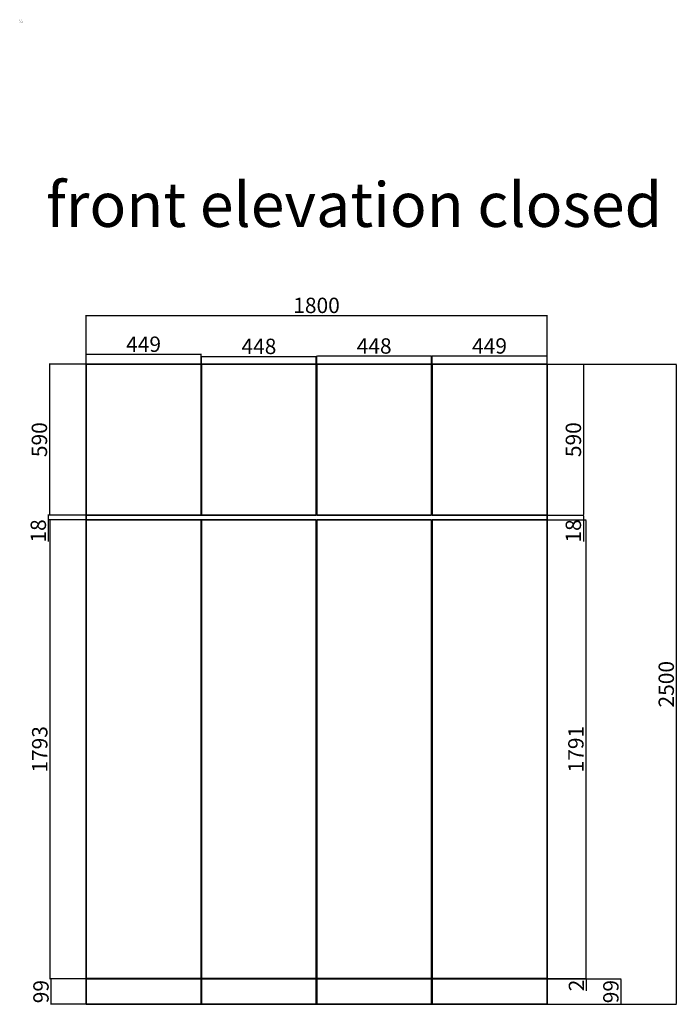
# Model space of a CAD drawing. Units: millimetres. Extents: x 222 to 5960, y 495 to 4622.
# Tile 3 of 3: x 3388 to 5960, y 776 to 4622. Entities that reach past the tile are written whole.
import ezdxf

# ---------------------------------------------------------------- set-up
doc = ezdxf.new("R2010")
doc.units = ezdxf.units.MM
for name, color, linetype, lineweight in [('A-ANNO-DIMS', 2, 'Continuous', 18), ('A-ANNO-TEXT', 3, 'Continuous', 25), ('A-FURN', 7, 'Continuous', 35)]:
    doc.layers.add(name, color=color, linetype=linetype, lineweight=lineweight)
doc.styles.get("Standard").update_dxf_attribs({"font": 'arial.ttf'})
doc.dimstyles.new('ISO-25', dxfattribs={"dimtxt": 60, "dimasz": 2.5, "dimexe": 1.25, "dimexo": 0.625, "dimtad": 1, "dimtxsty": 'Standard', "dimcen": 2.5, "dimadec": 0, "dimazin": 0, "dimtfac": 1, "dimtmove": 0, "dimatfit": 3, "dimfxl": 1, "dimarcsym": 0})

# ---------------------------------------------------------------- blocks, each defined once
blk = doc.blocks.new('*D38')
at = {"layer": 'A-ANNO-DIMS', "color": 0, "lineweight": -2, "transparency": 16777216}
for p, q in [((3647.7, 3277), (3647.7, 3316.4)), ((3650.2, 3315.2), (4094.2, 3315.2)), ((4096.7, 3277), (4096.7, 3316.4))]:
    blk.add_line(p, q, dxfattribs=at)
at = {"layer": 'A-ANNO-DIMS', "color": 0, "transparency": 16777216}
for points in [[(3650.2, 3315.6), (3650.2, 3314.8), (3647.7, 3315.2)], [(4094.2, 3315.6), (4094.2, 3314.8), (4096.7, 3315.2)]]:
    blk.add_solid(points, dxfattribs=at)
at = {"layer": 'Defpoints', "color": 0, "transparency": 16777216}
for p in [(4096.7, 3315.2), (3647.7, 3276.4), (4096.7, 3276.4)]:
    blk.add_point(p, dxfattribs=at)
at = {"layer": 'A-ANNO-DIMS', "color": 0, "transparency": 16777216, "insert": (3872.2, 3346.4), "char_height": 60, "attachment_point": 5}
blk.add_mtext('449', dxfattribs=at)
blk = doc.blocks.new('*D39')
at = {"layer": 'A-ANNO-DIMS', "color": 0, "lineweight": -2, "transparency": 16777216}
for p, q in [((4098.7, 3277), (4098.7, 3308)), ((4546.7, 3277), (4546.7, 3308)), ((4101.2, 3306.7), (4544.2, 3306.7))]:
    blk.add_line(p, q, dxfattribs=at)
at = {"layer": 'A-ANNO-DIMS', "color": 0, "transparency": 16777216}
for points in [[(4101.2, 3307.1), (4101.2, 3306.3), (4098.7, 3306.7)], [(4544.2, 3307.1), (4544.2, 3306.3), (4546.7, 3306.7)]]:
    blk.add_solid(points, dxfattribs=at)
at = {"layer": 'Defpoints', "color": 0, "transparency": 16777216}
for p in [(4098.7, 3276.4), (4546.7, 3306.7), (4546.7, 3276.4)]:
    blk.add_point(p, dxfattribs=at)
at = {"layer": 'A-ANNO-DIMS', "color": 0, "transparency": 16777216, "insert": (4322.7, 3338), "char_height": 60, "attachment_point": 5}
blk.add_mtext('448', dxfattribs=at)
blk = doc.blocks.new('*D40')
at = {"layer": 'A-ANNO-DIMS', "color": 0, "lineweight": -2, "transparency": 16777216}
for p, q in [((4548.7, 3277), (4548.7, 3309.4)), ((4551.2, 3308.2), (4994.2, 3308.2)), ((4996.7, 3277), (4996.7, 3309.4))]:
    blk.add_line(p, q, dxfattribs=at)
at = {"layer": 'A-ANNO-DIMS', "color": 0, "transparency": 16777216}
for points in [[(4551.2, 3308.6), (4551.2, 3307.8), (4548.7, 3308.2)], [(4994.2, 3308.6), (4994.2, 3307.8), (4996.7, 3308.2)]]:
    blk.add_solid(points, dxfattribs=at)
at = {"layer": 'Defpoints', "color": 0, "transparency": 16777216}
for p in [(4996.7, 3308.2), (4548.7, 3276.4), (4996.7, 3276.4)]:
    blk.add_point(p, dxfattribs=at)
at = {"layer": 'A-ANNO-DIMS', "color": 0, "transparency": 16777216, "insert": (4772.7, 3339.5), "char_height": 60, "attachment_point": 5}
blk.add_mtext('448', dxfattribs=at)
blk = doc.blocks.new('*D41')
at = {"layer": 'A-ANNO-DIMS', "color": 0, "lineweight": -2, "transparency": 16777216}
for p, q in [((4998.7, 3277), (4998.7, 3309.7)), ((5001.2, 3308.5), (5445.2, 3308.5)), ((5447.7, 3277), (5447.7, 3309.7))]:
    blk.add_line(p, q, dxfattribs=at)
at = {"layer": 'A-ANNO-DIMS', "color": 0, "transparency": 16777216}
for points in [[(5001.2, 3308.9), (5001.2, 3308.1), (4998.7, 3308.5)], [(5445.2, 3308.9), (5445.2, 3308.1), (5447.7, 3308.5)]]:
    blk.add_solid(points, dxfattribs=at)
at = {"layer": 'Defpoints', "color": 0, "transparency": 16777216}
for p in [(5447.7, 3308.5), (4998.7, 3276.4), (5447.7, 3276.4)]:
    blk.add_point(p, dxfattribs=at)
at = {"layer": 'A-ANNO-DIMS', "color": 0, "transparency": 16777216, "insert": (5223.2, 3339.7), "char_height": 60, "attachment_point": 5}
blk.add_mtext('449', dxfattribs=at)
blk = doc.blocks.new('*D42')
at = {"layer": 'A-ANNO-DIMS', "color": 0, "lineweight": -2, "transparency": 16777216}
for p, q in [((3647.7, 3277), (3647.7, 3468)), ((3650.2, 3466.7), (5445.2, 3466.7)), ((5447.7, 3277), (5447.7, 3468))]:
    blk.add_line(p, q, dxfattribs=at)
at = {"layer": 'A-ANNO-DIMS', "color": 0, "transparency": 16777216}
for points in [[(3650.2, 3467.1), (3650.2, 3466.3), (3647.7, 3466.7)], [(5445.2, 3467.1), (5445.2, 3466.3), (5447.7, 3466.7)]]:
    blk.add_solid(points, dxfattribs=at)
at = {"layer": 'Defpoints', "color": 0, "transparency": 16777216}
for p in [(5447.7, 3466.7), (3647.7, 3276.4), (5447.7, 3276.4)]:
    blk.add_point(p, dxfattribs=at)
at = {"layer": 'A-ANNO-DIMS', "color": 0, "transparency": 16777216, "insert": (4547.7, 3498), "char_height": 60, "attachment_point": 5}
blk.add_mtext('1800', dxfattribs=at)
blk = doc.blocks.new('*D43')
at = {"layer": 'A-ANNO-DIMS', "color": 0, "lineweight": -2, "transparency": 16777216}
for p, q in [((5448.4, 3276.4), (5591, 3276.4)), ((5589.7, 3273.9), (5589.7, 2688.9)), ((5448.4, 2686.4), (5591, 2686.4))]:
    blk.add_line(p, q, dxfattribs=at)
at = {"layer": 'A-ANNO-DIMS', "color": 0, "transparency": 16777216}
for points in [[(5589.3, 3273.9), (5590.2, 3273.9), (5589.7, 3276.4)], [(5589.3, 2688.9), (5590.2, 2688.9), (5589.7, 2686.4)]]:
    blk.add_solid(points, dxfattribs=at)
at = {"layer": 'Defpoints', "color": 0, "transparency": 16777216}
for p in [(5447.7, 3276.4), (5447.7, 2686.4), (5589.7, 2686.4)]:
    blk.add_point(p, dxfattribs=at)
at = {"layer": 'A-ANNO-DIMS', "color": 0, "transparency": 16777216, "insert": (5558.5, 2981.4), "char_height": 60, "attachment_point": 5, "rotation": 90}
blk.add_mtext('590', dxfattribs=at)
blk = doc.blocks.new('*D44')
at = {"layer": 'A-ANNO-DIMS', "color": 0, "lineweight": -2, "transparency": 16777216}
for p, q in [((5448.4, 2686.4), (5590.8, 2686.4)), ((5448.4, 2668.4), (5590.8, 2668.4)), ((5589.6, 2683.9), (5589.6, 2670.9)), ((5589.6, 2668.4), (5589.6, 2584.2))]:
    blk.add_line(p, q, dxfattribs=at)
at = {"layer": 'A-ANNO-DIMS', "color": 0, "transparency": 16777216}
for points in [[(5589.1, 2683.9), (5590, 2683.9), (5589.6, 2686.4)], [(5589.1, 2670.9), (5590, 2670.9), (5589.6, 2668.4)]]:
    blk.add_solid(points, dxfattribs=at)
at = {"layer": 'Defpoints', "color": 0, "transparency": 16777216}
for p in [(5447.7, 2686.4), (5447.7, 2668.4), (5589.6, 2668.4)]:
    blk.add_point(p, dxfattribs=at)
at = {"layer": 'A-ANNO-DIMS', "color": 0, "transparency": 16777216, "insert": (5558.3, 2625), "char_height": 60, "attachment_point": 5, "rotation": 90}
blk.add_mtext('18', dxfattribs=at)
blk = doc.blocks.new('*D45')
at = {"layer": 'A-ANNO-DIMS', "color": 0, "lineweight": -2, "transparency": 16777216}
for p, q in [((5448.4, 2668.4), (5600.7, 2668.4)), ((5599.4, 2665.9), (5599.4, 879.9)), ((5448.4, 877.4), (5600.7, 877.4))]:
    blk.add_line(p, q, dxfattribs=at)
at = {"layer": 'A-ANNO-DIMS', "color": 0, "transparency": 16777216}
for points in [[(5599, 2665.9), (5599.8, 2665.9), (5599.4, 2668.4)], [(5599, 879.9), (5599.8, 879.9), (5599.4, 877.4)]]:
    blk.add_solid(points, dxfattribs=at)
at = {"layer": 'Defpoints', "color": 0, "transparency": 16777216}
for p in [(5447.7, 2668.4), (5447.7, 877.4), (5599.4, 877.4)]:
    blk.add_point(p, dxfattribs=at)
at = {"layer": 'A-ANNO-DIMS', "color": 0, "transparency": 16777216, "insert": (5568.2, 1772.9), "char_height": 60, "attachment_point": 5, "rotation": 90}
blk.add_mtext('1791', dxfattribs=at)
blk = doc.blocks.new('*D46')
at = {"layer": 'A-ANNO-DIMS', "color": 0, "lineweight": -2, "transparency": 16777216}
for p, q in [((5448.4, 877.4), (5602.4, 877.4)), ((5448.4, 875.4), (5602.4, 875.4)), ((5601.2, 879.9), (5601.2, 882.4)), ((5601.2, 877.4), (5601.2, 875.4)), ((5601.2, 872.9), (5601.2, 829.4))]:
    blk.add_line(p, q, dxfattribs=at)
at = {"layer": 'A-ANNO-DIMS', "color": 0, "transparency": 16777216}
for points in [[(5600.7, 879.9), (5601.6, 879.9), (5601.2, 877.4)], [(5600.7, 872.9), (5601.6, 872.9), (5601.2, 875.4)]]:
    blk.add_solid(points, dxfattribs=at)
at = {"layer": 'Defpoints', "color": 0, "transparency": 16777216}
for p in [(5447.7, 877.4), (5447.7, 875.4), (5601.2, 875.4)]:
    blk.add_point(p, dxfattribs=at)
at = {"layer": 'A-ANNO-DIMS', "color": 0, "transparency": 16777216, "insert": (5570.4, 849.9), "char_height": 60, "attachment_point": 5, "rotation": 90}
blk.add_mtext('2', dxfattribs=at)
blk = doc.blocks.new('*D47')
at = {"layer": 'A-ANNO-DIMS', "color": 0, "lineweight": -2, "transparency": 16777216}
for p, q in [((5448.4, 875.4), (5737.4, 875.4)), ((5736.2, 872.9), (5736.2, 778.9)), ((5448.4, 776.4), (5737.4, 776.4))]:
    blk.add_line(p, q, dxfattribs=at)
at = {"layer": 'A-ANNO-DIMS', "color": 0, "transparency": 16777216}
for points in [[(5735.8, 872.9), (5736.6, 872.9), (5736.2, 875.4)], [(5735.8, 778.9), (5736.6, 778.9), (5736.2, 776.4)]]:
    blk.add_solid(points, dxfattribs=at)
at = {"layer": 'Defpoints', "color": 0, "transparency": 16777216}
for p in [(5447.7, 875.4), (5447.7, 776.4), (5736.2, 776.4)]:
    blk.add_point(p, dxfattribs=at)
at = {"layer": 'A-ANNO-DIMS', "color": 0, "transparency": 16777216, "insert": (5704.9, 825.9), "char_height": 60, "attachment_point": 5, "rotation": 90}
blk.add_mtext('99', dxfattribs=at)
blk = doc.blocks.new('*D48')
at = {"layer": 'A-ANNO-DIMS', "color": 0, "lineweight": -2, "transparency": 16777216}
for p, q in [((5448.4, 3276.4), (5953.6, 3276.4)), ((5952.3, 3273.9), (5952.3, 778.9)), ((5448.4, 776.4), (5953.6, 776.4))]:
    blk.add_line(p, q, dxfattribs=at)
at = {"layer": 'A-ANNO-DIMS', "color": 0, "transparency": 16777216}
for points in [[(5951.9, 3273.9), (5952.7, 3273.9), (5952.3, 3276.4)], [(5951.9, 778.9), (5952.7, 778.9), (5952.3, 776.4)]]:
    blk.add_solid(points, dxfattribs=at)
at = {"layer": 'Defpoints', "color": 0, "transparency": 16777216}
for p in [(5447.7, 3276.4), (5447.7, 776.4), (5952.3, 776.4)]:
    blk.add_point(p, dxfattribs=at)
at = {"layer": 'A-ANNO-DIMS', "color": 0, "transparency": 16777216, "insert": (5921.1, 2026.4), "char_height": 60, "attachment_point": 5, "rotation": 90}
blk.add_mtext('2500', dxfattribs=at)
blk = doc.blocks.new('*D49')
at = {"layer": 'A-ANNO-DIMS', "color": 0, "lineweight": -2, "transparency": 16777216}
for p, q in [((3647.1, 3276.4), (3503.2, 3276.4)), ((3504.4, 3273.9), (3504.4, 2688.9)), ((3647.1, 2686.4), (3503.2, 2686.4))]:
    blk.add_line(p, q, dxfattribs=at)
at = {"layer": 'A-ANNO-DIMS', "color": 0, "transparency": 16777216}
for points in [[(3504, 3273.9), (3504.9, 3273.9), (3504.4, 3276.4)], [(3504, 2688.9), (3504.9, 2688.9), (3504.4, 2686.4)]]:
    blk.add_solid(points, dxfattribs=at)
at = {"layer": 'Defpoints', "color": 0, "transparency": 16777216}
for p in [(3647.7, 3276.4), (3504.4, 2686.4), (3647.7, 2686.4)]:
    blk.add_point(p, dxfattribs=at)
at = {"layer": 'A-ANNO-DIMS', "color": 0, "transparency": 16777216, "insert": (3473.2, 2981.4), "char_height": 60, "attachment_point": 5, "rotation": 90}
blk.add_mtext('590', dxfattribs=at)
blk = doc.blocks.new('*D50')
at = {"layer": 'A-ANNO-DIMS', "color": 0, "lineweight": -2, "transparency": 16777216}
for p, q in [((3647.1, 2686.4), (3498.9, 2686.4)), ((3647.1, 2668.4), (3498.9, 2668.4)), ((3500.2, 2683.9), (3500.2, 2670.9)), ((3500.2, 2668.4), (3500.2, 2584.2))]:
    blk.add_line(p, q, dxfattribs=at)
at = {"layer": 'A-ANNO-DIMS', "color": 0, "transparency": 16777216}
for points in [[(3499.8, 2683.9), (3500.6, 2683.9), (3500.2, 2686.4)], [(3499.8, 2670.9), (3500.6, 2670.9), (3500.2, 2668.4)]]:
    blk.add_solid(points, dxfattribs=at)
at = {"layer": 'Defpoints', "color": 0, "transparency": 16777216}
for p in [(3500.2, 2668.4), (3647.7, 2686.4), (3647.7, 2668.4)]:
    blk.add_point(p, dxfattribs=at)
at = {"layer": 'A-ANNO-DIMS', "color": 0, "transparency": 16777216, "insert": (3468.9, 2625), "char_height": 60, "attachment_point": 5, "rotation": 90}
blk.add_mtext('18', dxfattribs=at)
blk = doc.blocks.new('*D51')
at = {"layer": 'A-ANNO-DIMS', "color": 0, "lineweight": -2, "transparency": 16777216}
for p, q in [((3647.1, 2668.4), (3504.6, 2668.4)), ((3505.9, 2665.9), (3505.9, 877.9)), ((3647.1, 875.4), (3504.6, 875.4))]:
    blk.add_line(p, q, dxfattribs=at)
at = {"layer": 'A-ANNO-DIMS', "color": 0, "transparency": 16777216}
for points in [[(3505.5, 2665.9), (3506.3, 2665.9), (3505.9, 2668.4)], [(3505.5, 877.9), (3506.3, 877.9), (3505.9, 875.4)]]:
    blk.add_solid(points, dxfattribs=at)
at = {"layer": 'Defpoints', "color": 0, "transparency": 16777216}
for p in [(3647.7, 2668.4), (3505.9, 875.4), (3647.7, 875.4)]:
    blk.add_point(p, dxfattribs=at)
at = {"layer": 'A-ANNO-DIMS', "color": 0, "transparency": 16777216, "insert": (3474.6, 1771.9), "char_height": 60, "attachment_point": 5, "rotation": 90}
blk.add_mtext('1793', dxfattribs=at)
blk = doc.blocks.new('*D52')
at = {"layer": 'A-ANNO-DIMS', "color": 0, "lineweight": -2, "transparency": 16777216}
for p, q in [((3647.1, 875.4), (3509.3, 875.4)), ((3510.6, 872.9), (3510.6, 778.9)), ((3647.1, 776.4), (3509.3, 776.4))]:
    blk.add_line(p, q, dxfattribs=at)
at = {"layer": 'A-ANNO-DIMS', "color": 0, "transparency": 16777216}
for points in [[(3510.2, 872.9), (3511, 872.9), (3510.6, 875.4)], [(3510.2, 778.9), (3511, 778.9), (3510.6, 776.4)]]:
    blk.add_solid(points, dxfattribs=at)
at = {"layer": 'Defpoints', "color": 0, "transparency": 16777216}
for p in [(3647.7, 875.4), (3510.6, 776.4), (3647.7, 776.4)]:
    blk.add_point(p, dxfattribs=at)
at = {"layer": 'A-ANNO-DIMS', "color": 0, "transparency": 16777216, "insert": (3479.3, 825.9), "char_height": 60, "attachment_point": 5, "rotation": 90}
blk.add_mtext('99', dxfattribs=at)

msp = doc.modelspace()

# ---------------------------------------------------------------- linework, layer by layer
at = {"layer": 'A-FURN'}
for p, q in [((3647.738, 3276.379), (5447.738, 3276.379)), ((3647.738, 776.379), (3647.738, 3276.379)), ((4096.738, 2686.379), (4096.738, 3276.379)), ((4098.738, 2686.379), (4098.738, 3276.379)), ((4546.738, 2686.379), (4546.738, 3276.379)), ((4548.738, 2686.379), (4548.738, 3276.379)), ((4996.738, 2686.379), (4996.738, 3276.379)), ((4998.738, 2686.379), (4998.738, 3276.379)), ((5447.738, 3276.379), (5447.738, 776.379)), ((3647.738, 2686.379), (4096.738, 2686.379)), ((3647.738, 2668.379), (4096.738, 2668.379)), ((4096.738, 877.379), (4096.738, 2668.379)), ((4098.738, 2686.379), (4546.738, 2686.379)), ((4098.738, 877.379), (4098.738, 2668.379)), ((4098.738, 2668.379), (4546.738, 2668.379)), ((4546.738, 877.379), (4546.738, 2668.379)), ((4548.738, 2686.379), (4996.738, 2686.379)), ((4548.738, 877.379), (4548.738, 2668.379)), ((4548.738, 2668.379), (4996.738, 2668.379)), ((4996.738, 877.379), (4996.738, 2668.379)), ((4998.738, 2686.379), (5447.738, 2686.379)), ((4998.738, 877.379), (4998.738, 2668.379)), ((4998.738, 2668.379), (5447.738, 2668.379)), ((3647.738, 877.379), (4096.738, 877.379)), ((3647.738, 875.379), (4096.738, 875.379)), ((4096.738, 776.379), (4096.738, 875.379)), ((4098.738, 877.379), (4546.738, 877.379)), ((4098.738, 776.379), (4098.738, 875.379)), ((4098.738, 875.379), (4546.738, 875.379)), ((4546.738, 776.379), (4546.738, 875.379)), ((4548.738, 877.379), (4996.738, 877.379)), ((4548.738, 776.379), (4548.738, 875.379)), ((4548.738, 875.379), (4996.738, 875.379)), ((4996.738, 776.379), (4996.738, 875.379)), ((4998.738, 877.379), (5447.738, 877.379)), ((4998.738, 776.379), (4998.738, 875.379)), ((4998.738, 875.379), (5447.738, 875.379)), ((5447.738, 776.379), (3647.738, 776.379))]:
    msp.add_line(p, q, dxfattribs=at)

# ---------------------------------------------------------------- texts
at = {"layer": 'A-ANNO-TEXT', "attachment_point": 1}
for s, width, gutter_width, insert, char_height in [('front Elevation mopen ', 19.12874, 12.5, (3388.342, 4621.257), 2.5), ('front elevation closed', 7449.3992, 869.625, (3491.643, 3986.205), 173.92497)]:
    msp.add_mtext_dynamic_manual_height_columns(s, width=width, gutter_width=gutter_width, heights=[0], dxfattribs=dict(at, insert=insert, char_height=char_height))

# ---------------------------------------------------------------- dimensions: what is measured, and where the dimension line sits
at = {"layer": 'A-ANNO-DIMS'}
for base, p1, p2, picture, middle in [((5447.738, 3466.712), (3647.738, 3276.379), (5447.738, 3276.379), '*D42', (4547.738, 3497.972)), ((4096.738, 3315.183), (3647.738, 3276.379), (4096.738, 3276.379), '*D38', (3872.238, 3346.443)), ((4546.738, 3306.723), (4098.738, 3276.379), (4546.738, 3276.379), '*D39', (4322.738, 3337.983)), ((4996.738, 3308.195), (4548.738, 3276.379), (4996.738, 3276.379), '*D40', (4772.738, 3339.454)), ((5447.738, 3308.488), (4998.738, 3276.379), (5447.738, 3276.379), '*D41', (5223.238, 3339.747))]:
    dim = msp.add_linear_dim(base=base, p1=p1, p2=p2, dimstyle='ISO-25', override={"dimclrd": 0, "dimclre": 0, "dimclrt": 0}, dxfattribs=at)
    dim.commit()
    dim.dimension.update_dxf_attribs({"geometry": picture, "text_midpoint": middle})
for base, p1, p2, picture, middle in [((3504.446, 2686.379), (3647.738, 3276.379), (3647.738, 2686.379), '*D49', (3473.187, 2981.379)), ((5589.736, 2686.379), (5447.738, 3276.379), (5447.738, 2686.379), '*D43', (5558.477, 2981.379)), ((5952.312, 776.379), (5447.738, 3276.379), (5447.738, 776.379), '*D48', (5921.053, 2026.379)), ((3500.187, 2668.379), (3647.738, 2686.379), (3647.738, 2668.379), '*D50', (3468.928, 2625.043)), ((3505.869, 875.379), (3647.738, 2668.379), (3647.738, 875.379), '*D51', (3474.589, 1771.879)), ((5589.566, 2668.379), (5447.738, 2686.379), (5447.738, 2668.379), '*D44', (5558.306, 2625.043)), ((5599.423, 877.379), (5447.738, 2668.379), (5447.738, 877.379), '*D45', (5568.163, 1772.879)), ((3510.582, 776.379), (3647.738, 875.379), (3647.738, 776.379), '*D52', (3479.323, 825.879)), ((5601.166, 875.379), (5447.738, 877.379), (5447.738, 875.379), '*D46', (5570.418, 849.884)), ((5736.186, 776.379), (5447.738, 875.379), (5447.738, 776.379), '*D47', (5704.926, 825.879))]:
    dim = msp.add_linear_dim(base=base, p1=p1, p2=p2, angle=90, dimstyle='ISO-25', override={"dimclrd": 0, "dimclre": 0, "dimclrt": 0}, dxfattribs=at)
    dim.commit()
    dim.dimension.update_dxf_attribs({"geometry": picture, "text_midpoint": middle})

doc.saveas('drawing.dxf')
